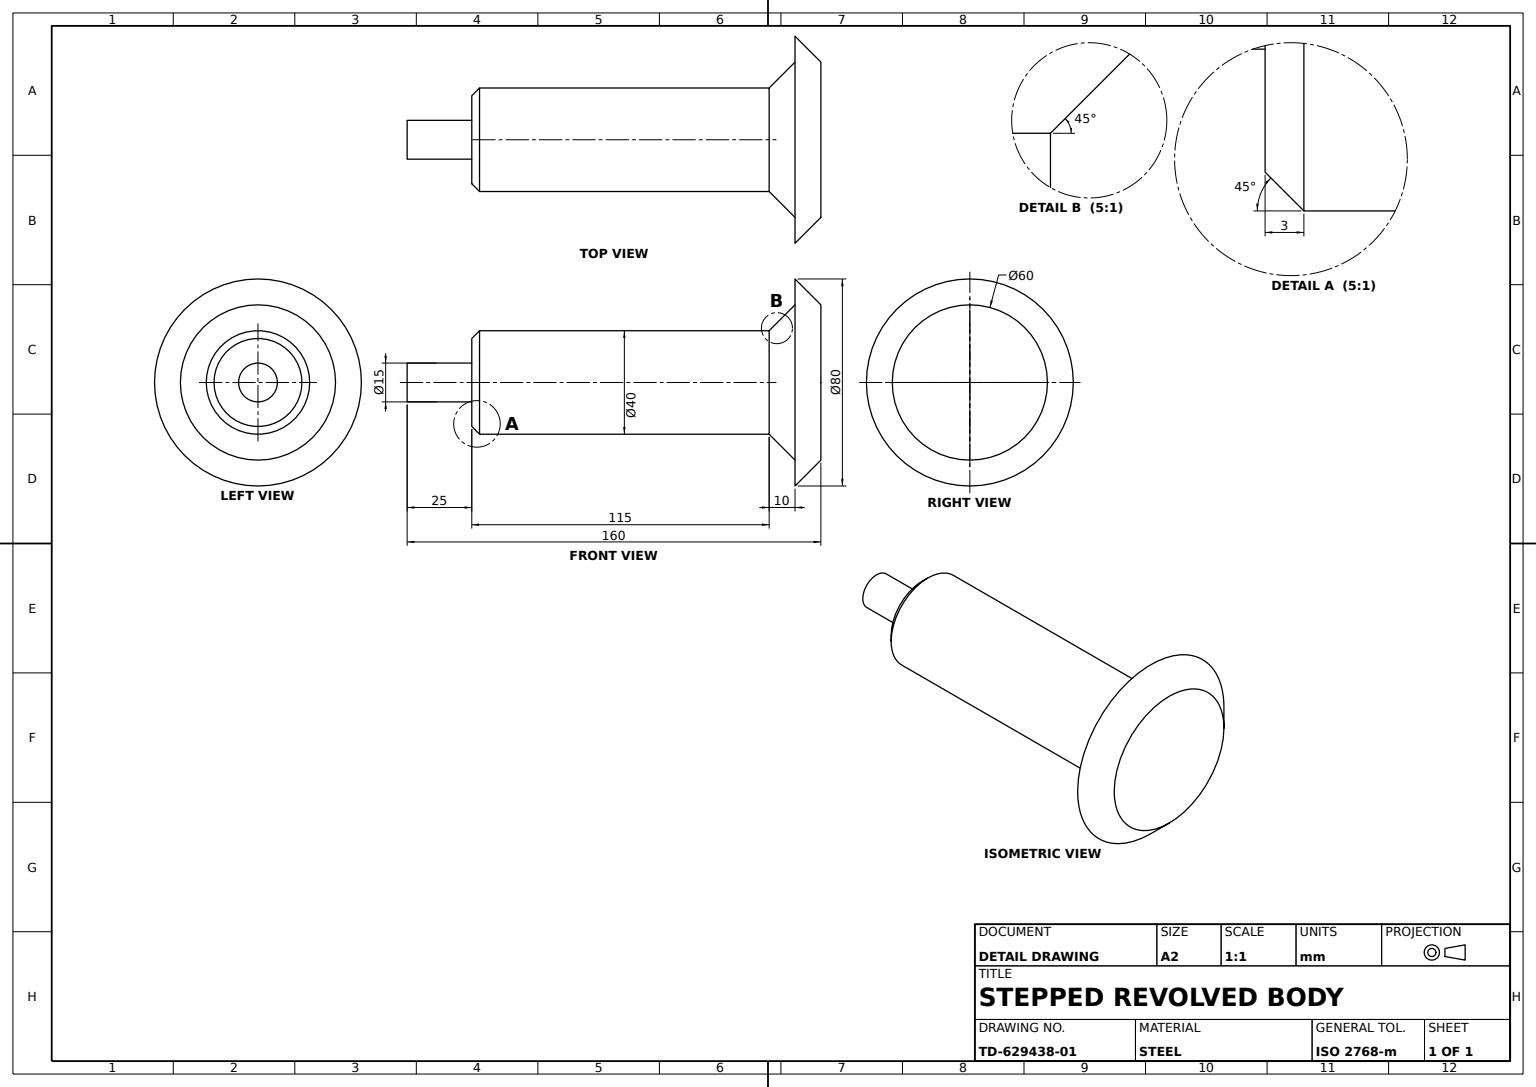
from build123d import *

# Parameters (mm, degrees)
PLUNGER_PROFILE_SKETCH_W   = 25
PLUNGER_PROFILE_SKETCH_H   = 7.5
PLUNGER_PROFILE_SKETCH_W_2 = 112
PLUNGER_PROFILE_SKETCH_H_2 = 20


with BuildPart() as part:
    # Plunger Profile Sketch → Plunger Body Revolve (revolve)
    with BuildSketch(Plane.XY, mode=Mode.PRIVATE) as plunger_body_revolve_sk:
        with Locations((-23.33175597, 3.75)):
            Rectangle(PLUNGER_PROFILE_SKETCH_W, PLUNGER_PROFILE_SKETCH_H)
        Polygon((-10.83175597, 7.5), (-10.83175597, 0), (-7.83175597, 0), (-7.83175597, 20), (-10.83175597, 17), align=None)
        with Locations((48.16824403, 10)):
            Rectangle(PLUNGER_PROFILE_SKETCH_W_2, PLUNGER_PROFILE_SKETCH_H_2)
        Polygon((104.16824403, 20), (104.16824403, 0), (114.16824403, 0), (114.16824403, 30), align=None)
        Polygon((114.16824403, 30), (114.16824403, 0), (124.16824403, 0), (124.16824403, 30), (114.16824403, 40), align=None)
    revolve(plunger_body_revolve_sk.sketch.rotate(Axis((-51.8095123, 0, 0), (1, 0, 0)), 90), axis=Axis((-51.8095123, 0, 0), (1, 0, 0)))


solid = part.part
